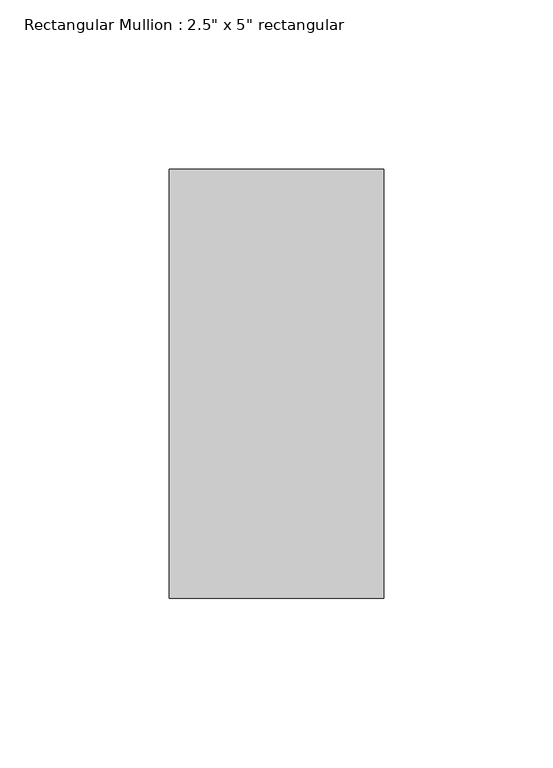
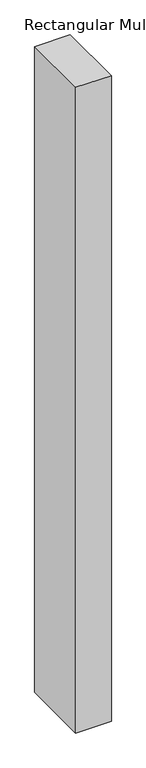
"""IFC4 building model written with IfcOpenShell, lengths in millimetres: member geometry."""

from ifc_helpers import new_model, si_unit, frame, origin, place, context, project, spatial, polyline, outline, extrude, source, transform, mapped, element, save


def member_75074519(model_context):
    return source(origin(), model_context, "Body", "SweptSolid", [
        extrude(outline(polyline([(0.0, 63.5), (0.0, -63.5), (-63.5, -63.5), (-63.5, 63.5), (0.0, 63.5)])), frame((0.0, 0.0, -1219.2), z_axis=(0.0, 0.0, 1.0), x_axis=(1.0, 0.0, 0.0)), (0.0, 0.0, 1.0), 1219.2),
    ])


if __name__ == "__main__":
    model = new_model("IFC4")
    model_context = context("Model", 3, world=origin())
    ifc_project = project(units=[si_unit("LENGTHUNIT", "METRE", prefix="MILLI")], contexts=[model_context])
    site = spatial("IfcSite", under=ifc_project)
    building = spatial("IfcBuilding", under=site)
    placement = place(None, origin())
    member_shape = member_75074519(model_context)
    element("IfcMember", 1, ObjectType="Rectangular Mullion : 2.5\" x 5\" rectangular", at=placement, inside=building, context=model_context, shape_type="MappedRepresentation", body=[
        mapped(member_shape, transform((0.0, 0.0, 0.0), x_axis=(1.0, 0.0, 0.0), y_axis=(0.0, 1.0, 0.0), z_axis=(0.0, 0.0, 1.0))),
    ])
    save(model, "model.ifc")

# Revit data of these elements
# Type "Rectangular Mullion : 2.5\" x 5\" rectangular"
#   built-in parameter 1007304 = 0.416667 (stored number, unit not read)
#   built-in parameter 1007301 = 0.104167 (stored number, unit not read)
#   built-in parameter 1007300 = 0.104167 (stored number, unit not read)
# Element 1 (IfcMember, "Rectangular Mullion : 2.5\" x 5\" rectangular")
#   Materials on its faces: "metal black"
# Materials
#   "metal black": class "Generic", colour RGB 120 120 120, transparency 0, Cost = 0
